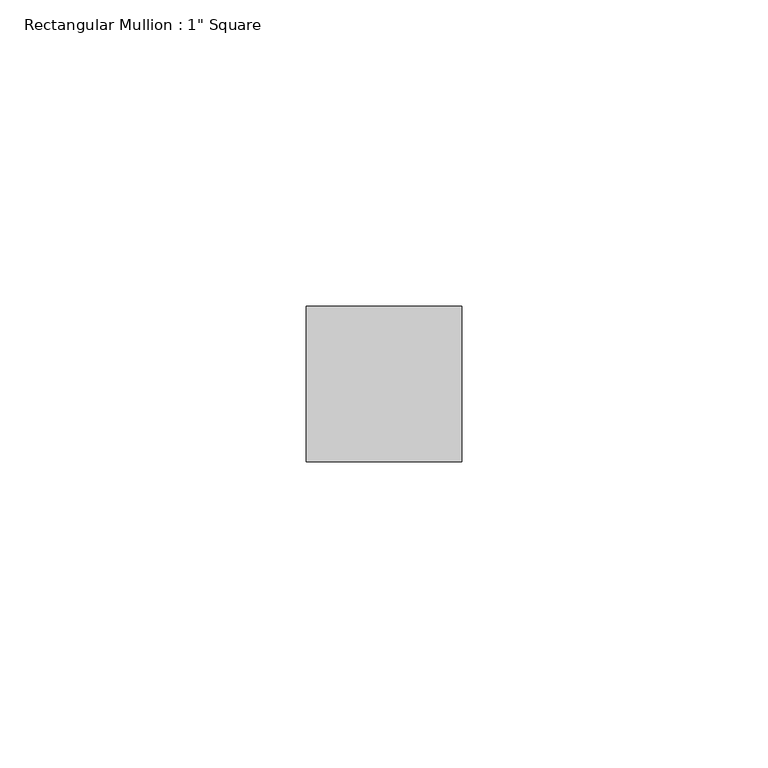
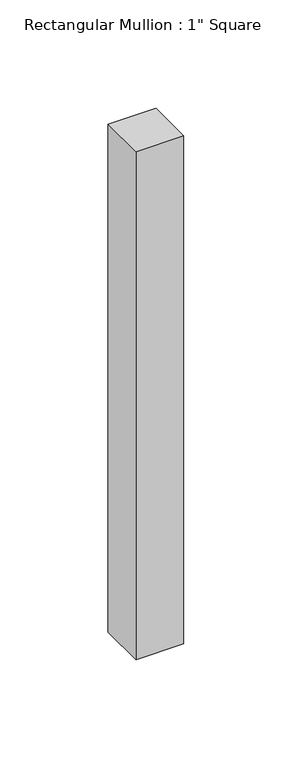
"""IFC4 building model written with IfcOpenShell, lengths in millimetres: member geometry."""

from ifc_helpers import new_model, si_unit, frame, origin, place, context, project, spatial, polyline, outline, extrude, source, transform, mapped, element, save


def member_fa046a42(model_context):
    return source(origin(), model_context, "Body", "SweptSolid", [
        extrude(outline(polyline([(12.7, 12.7), (12.7, -12.7), (-12.7, -12.7), (-12.7, 12.7), (12.7, 12.7)])), frame((0.0, 0.0, -285.75), z_axis=(0.0, 0.0, 1.0), x_axis=(1.0, 0.0, 0.0)), (0.0, 0.0, 1.0), 285.75),
    ])


if __name__ == "__main__":
    model = new_model("IFC4")
    model_context = context("Model", 3, world=origin())
    ifc_project = project(units=[si_unit("LENGTHUNIT", "METRE", prefix="MILLI")], contexts=[model_context])
    site = spatial("IfcSite", under=ifc_project)
    building = spatial("IfcBuilding", under=site)
    placement = place(None, origin())
    member_shape = member_fa046a42(model_context)
    element("IfcMember", 1, ObjectType="Rectangular Mullion : 1\" Square", at=placement, inside=building, context=model_context, shape_type="MappedRepresentation", body=[
        mapped(member_shape, transform((0.0, 0.0, 0.0), x_axis=(1.0, 0.0, 0.0), y_axis=(0.0, 1.0, 0.0), z_axis=(0.0, 0.0, 1.0))),
    ])
    save(model, "model.ifc")

# Revit data of these elements
# Type "Rectangular Mullion : 1\" Square"
#   built-in parameter 1007304 = 0.0833333 (stored number, unit not read)
#   built-in parameter 1007301 = 0.0416667 (stored number, unit not read)
#   built-in parameter 1007300 = 0.0416667 (stored number, unit not read)
# Element 1 (IfcMember, "Rectangular Mullion : 1\" Square")
#   Materials on its faces: "Aluminum"
# Materials
#   "Aluminum": class "Metal", colour RGB 247 247 247, transparency 0, Description = "Aluminum 6061", Cost = 0
